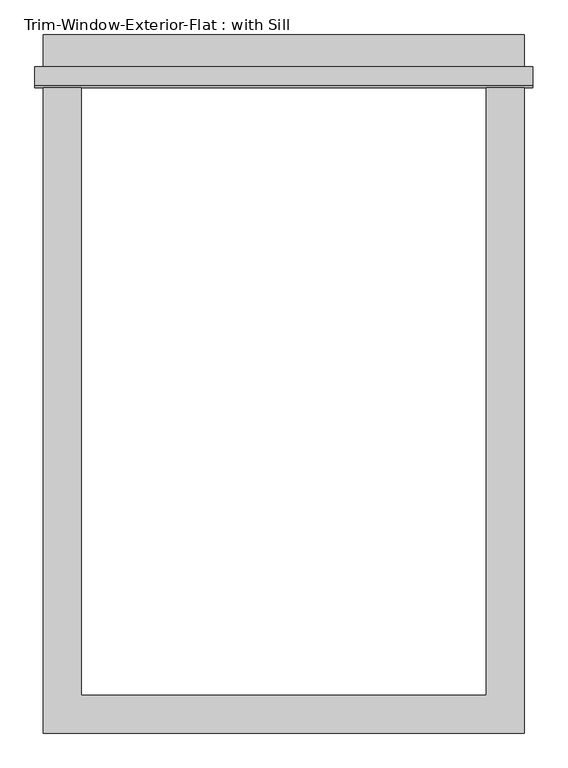
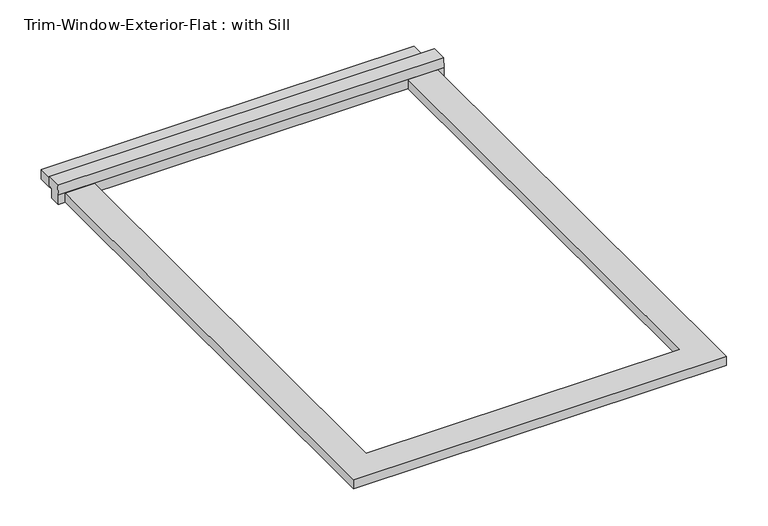
"""IFC4 building model written with IfcOpenShell, lengths in millimetres: proxy geometry, Trim-Window-Exterior-Flat : with Sill."""

from ifc_helpers import new_model, si_unit, frame, origin, origin_with_axes, place, context, project, spatial, polyline, outline, extrude, source, transform, mapped, element, save


def trim_window_exterior_flat_with_sill_4c72db77(model_context):
    return source(origin(), model_context, "Body", "SweptSolid", [
        extrude(outline(polyline([(361.95, 936.5823709), (-361.95, 936.5823709), (-361.95, 993.7323709), (361.95, 993.7323709), (361.95, 936.5823709)])), origin_with_axes(), (0.0, 0.0, 1.0), 19.05),
        extrude(outline(polyline([(946.15, 38.1), (946.15, 19.05), (936.5823709, 19.05), (936.5823709, 0.0), (914.4, 0.0), (914.4, 19.05), (916.8580645, 38.1), (946.15, 38.1)])), frame((-374.65, 0.0, 0.0), z_axis=(1.0, 0.0, 0.0), x_axis=(0.0, 1.0, 0.0)), (0.0, 0.0, 1.0), 749.3),
        extrude(outline(polyline([(-361.95, -57.15), (-361.95, 914.4), (-304.8, 914.4), (-304.8, 0.0), (304.8, 0.0), (304.8, 914.4), (361.95, 914.4), (361.95, -57.15), (-361.95, -57.15)])), origin_with_axes(), (0.0, 0.0, 1.0), 19.05),
    ])


if __name__ == "__main__":
    model = new_model("IFC4")
    model_context = context("Model", 3, world=origin())
    ifc_project = project(units=[si_unit("LENGTHUNIT", "METRE", prefix="MILLI")], contexts=[model_context])
    site = spatial("IfcSite", under=ifc_project)
    building = spatial("IfcBuilding", under=site)
    placement = place(None, origin())
    trim_window_exterior_flat_with_sill_shape = trim_window_exterior_flat_with_sill_4c72db77(model_context)
    element("IfcBuildingElementProxy", 1, Name="Trim-Window-Exterior-Flat : with Sill", ObjectType="Trim-Window-Exterior-Flat : with Sill", at=placement, inside=building, context=model_context, shape_type="MappedRepresentation", body=[
        mapped(trim_window_exterior_flat_with_sill_shape, transform((0.0, 0.0, 0.0), x_axis=(1.0, 0.0, 0.0), y_axis=(0.0, 1.0, 0.0), z_axis=(0.0, 0.0, 1.0))),
    ])
    save(model, "model.ifc")

# Revit data of these elements
# Type "Trim-Window-Exterior-Flat : with Sill"
#   Trim Width = 0' - 2 1/4"
#   Trim Thickness_Picture Frame = 0' - 1 1/4"
#   Trim Thickness_with Sill = 0' - 0 3/4"
#   Sill Thickness = 0' - 1 1/4"
#   Opening Width [instance default] = 2' - 0"
#   Opening Height [instance default] = 3' - 0"
#   Default Elevation = 4' - 0"
#   Sill = yes
#   Picture Frame = no
#   Trim Material [instance default] = none
# Element 1 (IfcBuildingElementProxy, "Trim-Window-Exterior-Flat : with Sill")
#   Trim Material = Clad - White
#   Materials on its faces: "Clad - White"
# Materials
#   "Clad - White": class "Wood", colour RGB 242 242 238, transparency 0, Cost = 0
